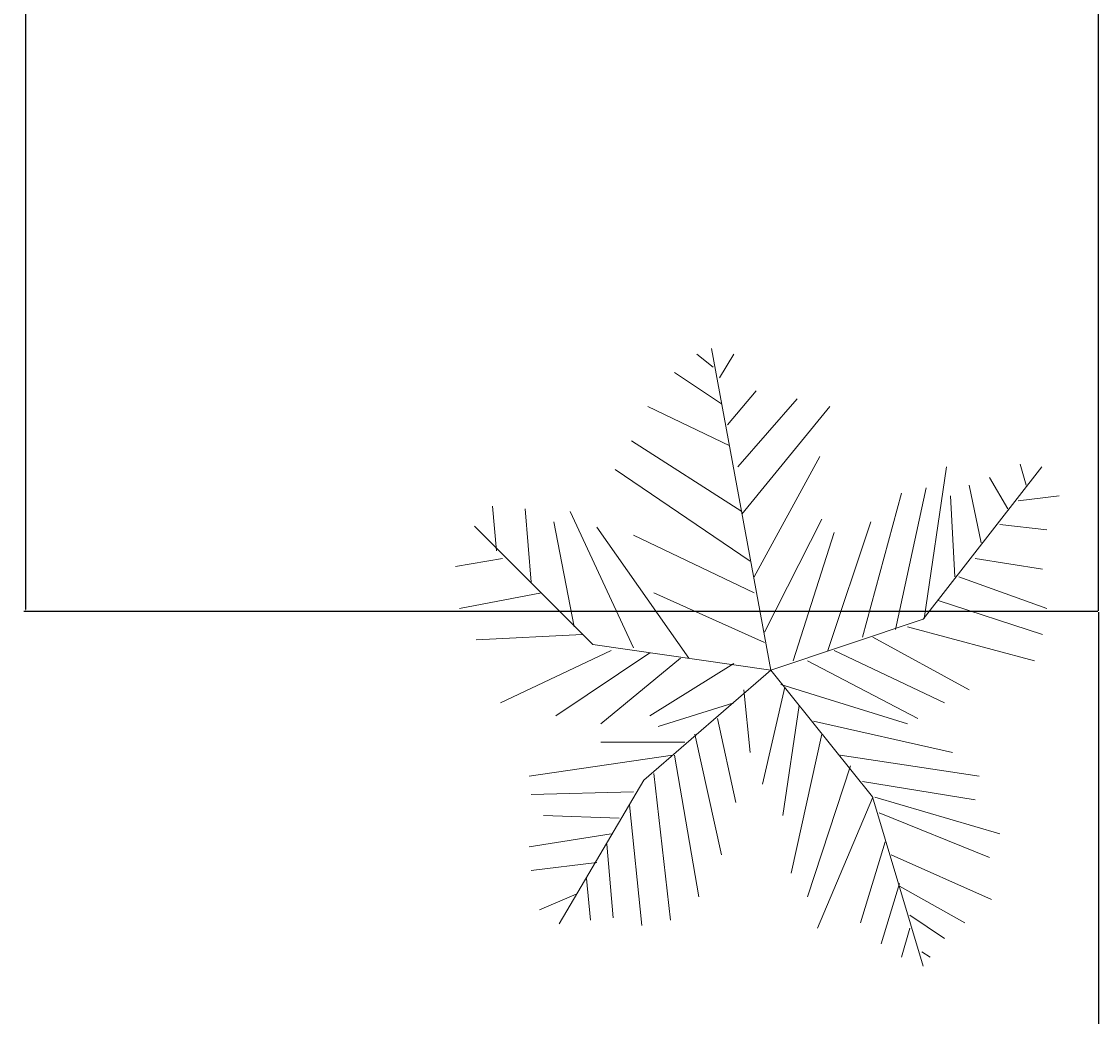
# Model space of a CAD drawing. Units: inches. Extents: x -301 to 715, y -607 to 364.
# Tile 52 of 141: x -301 to -205, y -260 to -171. Entities that reach past the tile are written whole.
import ezdxf

# ---------------------------------------------------------------- set-up
doc = ezdxf.new("R2010")
doc.units = ezdxf.units.IN
doc.header["$MEASUREMENT"] = 0
doc.layers.add('A-ANNO-DIMS', color=2, linetype='Continuous', lineweight=18)
doc.layers.add('L-PLNT', color=94, linetype='Continuous', lineweight=13)
doc.styles.get("Standard").update_dxf_attribs({"font": 'arial.ttf'})
doc.dimstyles.get("Standard").update_dxf_attribs({"dimtxt": 0.18, "dimasz": 0.18, "dimexe": 0.18, "dimexo": 0.0625, "dimgap": 0.09, "dimtad": 0, "dimtih": 1, "dimtoh": 1, "dimdec": 1, "dimzin": 0, "dimdsep": 46, "dimlunit": 4, "dimtxsty": 'Standard', "dimcen": 0.09, "dimclrd": 3, "dimclre": 4, "dimclrt": 6, "dimadec": 0, "dimazin": 0, "dimtfac": 1, "dimtdec": 1, "dimtofl": 0, "dimtmove": 0, "dimatfit": 3, "dimfxl": 1, "dimtfill": 2, "dimtfillclr": 51, "dimtolj": 1, "dimtzin": 0, "dimarcsym": 0})

# ---------------------------------------------------------------- blocks, each defined once
blk = doc.blocks.new('*U33')
for p, q in [((-10.186, 53.64), (-13.084, 55.962)), ((0, 0), (-10.5, 57)), ((-9.099, 51.782), (-6.563, 55.962)), ((-8.737, 47.138), (-17.069, 52.711)), ((-7.65, 43.423), (-2.578, 49.46)), ((-5.839, 35.992), (4.667, 48.067)), ((-7.288, 39.707), (-21.778, 46.673)), ((-5.114, 27.632), (10.463, 46.673)), ((-5.114, 28.097), (-24.676, 40.636)), ((-2.941, 16.486), (8.652, 37.85)), ((44.153, 36.456), (45.239, 32.741)), ((-3.665, 19.273), (-27.574, 35.527)), ((27, 9), (48, 36)), ((27.127, 9.056), (31.112, 35.992)), ((35.096, 32.741), (37.27, 22.524)), ((38.719, 34.134), (41.979, 28.561)), ((16.259, 5.805), (23.142, 31.348)), ((22.055, 7.198), (27.489, 32.277)), ((31.836, 30.883), (32.561, 16.486)), ((43.791, 29.954), (51.036, 30.883)), ((-48.585, 21.131), (-49.309, 29.026)), ((-43.513, 28.561), (-42.427, 15.558)), ((-35.544, 28.097), (-24.314, 3.947)), ((-1.129, 6.734), (9.014, 26.704)), ((-31.5, 4.5), (-52.5, 25.5)), ((-38.442, 26.239), (-34.819, 7.663)), ((-14.533, 2.09), (-30.834, 25.31)), ((10.101, 3.483), (17.708, 26.239)), ((40.53, 25.775), (48.862, 24.846)), ((-24.314, 23.917), (-2.941, 13.7)), ((3.942, 1.625), (11.187, 24.381)), ((-47.498, 19.737), (-55.83, 18.344)), ((36.183, 19.737), (48.137, 17.88)), ((33.285, 16.486), (48.862, 10.913)), ((-40.615, 13.7), (-55.105, 10.913)), ((-20.691, 13.7), (-1.129, 4.876)), ((29.662, 12.307), (48.137, 6.269)), ((0, 0), (27, 9)), ((24.229, 7.663), (46.688, 1.625)), ((-33.37, 6.269), (-52.207, 5.34)), ((18.07, 5.805), (35.096, -3.483)), ((0, 0), (-31.5, 4.5)), ((-28.299, 3.483), (-47.86, -5.805)), ((-21.416, 3.018), (-38.079, -8.128)), ((-15.982, 2.09), (-30.11, -9.521)), ((11.187, 3.483), (30.749, -5.805)), ((0, 0), (-22.5, -19.5)), ((-6.563, 1.161), (-21.416, -8.128)), ((0, 0), (18, -22.5)), ((6.478, 1.625), (26.04, -8.592)), ((-4.752, -3.483), (-3.665, -14.629)), ((2.493, -3.019), (-1.491, -20.202)), ((1.769, -2.555), (24.229, -9.521)), ((-6.563, -5.805), (-19.967, -9.985)), ((5.029, -6.27), (2.131, -25.775)), ((-9.461, -8.592), (-6.201, -23.453)), ((7.565, -9.056), (32.198, -14.629)), ((-13.446, -11.378), (-8.737, -32.741)), ((9.014, -11.378), (3.58, -35.992)), ((-15.257, -12.772), (-30.11, -12.772)), ((-17.431, -15.094), (-42.789, -18.809)), ((-17.069, -15.094), (-12.721, -40.172)), ((12.274, -15.094), (36.907, -18.809)), ((14.085, -16.951), (6.478, -40.172)), ((-20.691, -18.345), (-17.793, -44.352)), ((-22.5, -19.5), (-37.5, -45)), ((16.259, -19.738), (36.183, -22.989)), ((-24.314, -21.596), (-42.427, -22.06)), ((18.07, -22.524), (8.289, -45.745)), ((18, -22.5), (27, -52.5)), ((18.433, -22.524), (40.53, -29.026)), ((-25.038, -23.918), (-22.865, -45.281)), ((-26.849, -26.24), (-40.253, -25.775)), ((19.157, -25.311), (38.719, -33.206)), ((-28.299, -29.026), (-42.789, -31.348)), ((20.244, -30.419), (15.897, -44.816)), ((-29.023, -30.884), (-27.936, -43.887)), ((-30.834, -34.135), (-42.427, -35.528)), ((21.331, -32.741), (39.081, -40.636)), ((-32.646, -36.921), (-31.921, -44.352)), ((22.78, -37.85), (19.519, -48.532)), ((-34.457, -39.708), (-40.978, -42.494)), ((22.78, -38.314), (34.372, -44.816)), ((24.591, -43.423), (30.749, -47.603)), ((24.591, -45.745), (23.142, -50.854)), ((26.764, -49.925), (28.213, -50.854))]:
    blk.add_line(p, q)
blk = doc.blocks.new('*D145')
at = {"layer": 'A-ANNO-DIMS', "color": 4, "lineweight": -2, "transparency": 16777216}
for p, q in [((-204.666, 310.182), (-300.87, 310.182)), ((-204.666, -223.818), (-300.87, -223.818))]:
    blk.add_line(p, q, dxfattribs=at)
at = {"layer": 'A-ANNO-DIMS', "color": 3, "lineweight": -2, "transparency": 16777216}
for p, q in [((-300.69, 310.002), (-300.69, 43.364)), ((-300.69, -223.638), (-300.69, 43))]:
    blk.add_line(p, q, dxfattribs=at)
at = {"layer": 'A-ANNO-DIMS', "color": 3, "transparency": 16777216}
for points in [[(-300.72, 310.002), (-300.66, 310.002), (-300.69, 310.182)], [(-300.72, -223.638), (-300.66, -223.638), (-300.69, -223.818)]]:
    blk.add_solid(points, dxfattribs=at)
at = {"layer": 'Defpoints', "color": 0, "transparency": 16777216}
for p in [(-300.69, 310.182), (-204.603, 310.182), (-204.603, -223.818)]:
    blk.add_point(p, dxfattribs=at)
at = {"layer": 'A-ANNO-DIMS', "color": 6, "transparency": 16777216, "insert": (-300.69, 43.182), "char_height": 0.18, "attachment_point": 5, "bg_fill": 1, "box_fill_scale": 1.25, "bg_fill_color": 51, "bg_fill_transparency": 0}
blk.add_mtext('\\A1;44\'-6"', dxfattribs=at)
blk = doc.blocks.new('*D146')
at = {"layer": 'A-ANNO-DIMS', "color": 4, "lineweight": -2, "transparency": 16777216}
for p, q in [((-204.603, -223.88), (-204.603, -296.865)), ((-143.603, -223.88), (-143.603, -296.865))]:
    blk.add_line(p, q, dxfattribs=at)
at = {"layer": 'A-ANNO-DIMS', "color": 3, "lineweight": -2, "transparency": 16777216}
for p, q in [((-204.423, -296.685), (-174.433, -296.685)), ((-143.783, -296.685), (-173.774, -296.685))]:
    blk.add_line(p, q, dxfattribs=at)
at = {"layer": 'A-ANNO-DIMS', "color": 3, "transparency": 16777216}
for points in [[(-204.423, -296.655), (-204.423, -296.715), (-204.603, -296.685)], [(-143.783, -296.655), (-143.783, -296.715), (-143.603, -296.685)]]:
    blk.add_solid(points, dxfattribs=at)
at = {"layer": 'Defpoints', "color": 0, "transparency": 16777216}
for p in [(-204.603, -223.818), (-143.603, -223.818), (-143.603, -296.685)]:
    blk.add_point(p, dxfattribs=at)
at = {"layer": 'A-ANNO-DIMS', "color": 6, "transparency": 16777216, "insert": (-174.103, -296.685), "char_height": 0.18, "attachment_point": 5, "bg_fill": 1, "box_fill_scale": 1.25, "bg_fill_color": 51, "bg_fill_transparency": 0}
blk.add_mtext('\\A1;5\'-1"', dxfattribs=at)
blk = doc.blocks.new('*D151')
at = {"layer": 'A-ANNO-DIMS', "color": 4, "lineweight": -2, "transparency": 16777216}
for p, q in [((-204.603, -223.755), (-204.603, 359.612)), ((-45.603, -214.755), (-45.603, 359.612))]:
    blk.add_line(p, q, dxfattribs=at)
at = {"layer": 'A-ANNO-DIMS', "color": 3, "lineweight": -2, "transparency": 16777216}
for p, q in [((-204.423, 359.432), (-125.494, 359.432)), ((-45.783, 359.432), (-124.713, 359.432))]:
    blk.add_line(p, q, dxfattribs=at)
at = {"layer": 'A-ANNO-DIMS', "color": 3, "transparency": 16777216}
for points in [[(-204.423, 359.462), (-204.423, 359.402), (-204.603, 359.432)], [(-45.783, 359.462), (-45.783, 359.402), (-45.603, 359.432)]]:
    blk.add_solid(points, dxfattribs=at)
at = {"layer": 'Defpoints', "color": 0, "transparency": 16777216}
for p in [(-45.603, 359.432), (-45.603, -214.818), (-204.603, -223.818)]:
    blk.add_point(p, dxfattribs=at)
at = {"layer": 'A-ANNO-DIMS', "color": 6, "transparency": 16777216, "insert": (-125.103, 359.432), "char_height": 0.18, "attachment_point": 5, "bg_fill": 1, "box_fill_scale": 1.25, "bg_fill_color": 51, "bg_fill_transparency": 0}
blk.add_mtext('\\A1;13\'-3"', dxfattribs=at)

msp = doc.modelspace()

# ---------------------------------------------------------------- block references
at = {"layer": 'L-PLNT', "xscale": 0.5058896831792554, "yscale": 0.5058896831792554, "zscale": 0.5058896831792554}
msp.add_blockref('*U33', (-233.954, -229.069), dxfattribs=at)

# ---------------------------------------------------------------- dimensions: what is measured, and where the dimension line sits
at = {"layer": 'A-ANNO-DIMS'}
for base, p2, picture, middle in [((-45.603, 359.432), (-45.603, -214.818), '*D151', (-125.103, 359.432)), ((-143.603, -296.685), (-143.603, -223.818), '*D146', (-174.103, -296.685))]:
    dim = msp.add_linear_dim(base=base, p1=(-204.603, -223.818), p2=p2, dimstyle='Standard', override={"dimdec": 1, "dimlfac": 1, "dimrnd": 0, "dimzin": 1, "dimdsep": 46, "dimlunit": 4, "dimfrac": 2}, dxfattribs=at)
    dim.commit()
    dim.dimension.update_dxf_attribs({"geometry": picture, "text_midpoint": middle})
dim = msp.add_linear_dim(base=(-300.69, 310.182), p1=(-204.603, -223.818), p2=(-204.603, 310.182), angle=90, dimstyle='Standard', override={"dimdec": 1, "dimlfac": 1, "dimrnd": 0, "dimzin": 1, "dimdsep": 46, "dimlunit": 4, "dimfrac": 2}, dxfattribs=at)
dim.commit()
dim.dimension.update_dxf_attribs({"geometry": '*D145', "text_midpoint": (-300.69, 43.182)})

doc.saveas('drawing.dxf')
